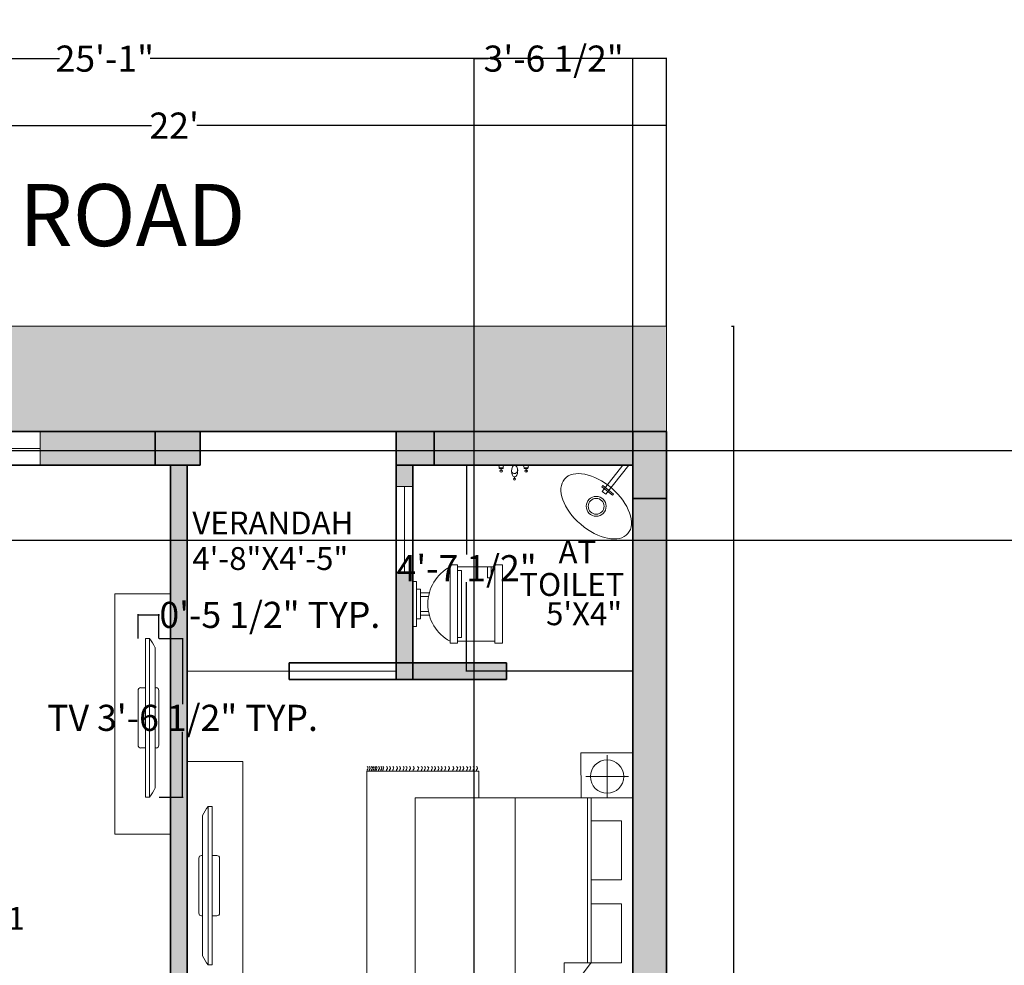
# Model space of a CAD drawing. Units: inches. Extents: x -17 to 892, y -721 to 172.
# Tile 6 of 11: x 174 to 438, y -82 to 172. Entities that reach past the tile are written whole.
import ezdxf

# ---------------------------------------------------------------- set-up
doc = ezdxf.new("R2010")
doc.units = ezdxf.units.IN
doc.header["$MEASUREMENT"] = 0
doc.layers.get('0').update_dxf_attribs({"color": 14})
for name, color, linetype, lineweight in [('A-ANNO-DIMS', 2, 'Continuous', 18), ('A-ANNO-TEXT', 7, 'Continuous', 18), ('A-AREA-IDEN', 7, 'Continuous', 18), ('A-COLS', 252, 'Continuous', 35), ('A-EQPM', 8, 'Continuous', 18), ('A-FLOR-CASE', 252, 'Continuous', 18), ('A-FLOR-FIXT', 8, 'Continuous', 18), ('A-WALL-PATT', 14, 'Continuous', 13), ('C-ROAD', 8, 'Continuous', 18), ('doors', 4, 'Continuous', 18), ('furniture', 252, 'Continuous', 18), ('walls', 252, 'Continuous', 35), ('windows', 161, 'Continuous', 18)]:
    doc.layers.add(name, color=color, linetype=linetype, lineweight=lineweight)
doc.layers.add('A-COLS-PATT', color=254, linetype='Continuous', lineweight=13, true_color=0xd7ebd2)
doc.layers.add('C-ROAD-PATT', color=9, linetype='Continuous', lineweight=13, true_color=0xafd9aa)
doc.styles.get("Standard").update_dxf_attribs({"font": 'arial.ttf'})
doc.dimstyles.get("Standard").update_dxf_attribs({"dimtxt": 7, "dimasz": 0.18, "dimexe": 0.18, "dimexo": 0.0625, "dimgap": 0.09, "dimtad": 0, "dimtih": 1, "dimtoh": 1, "dimzin": 0, "dimdsep": 46, "dimlunit": 3, "dimtxsty": 'Standard', "dimcen": 0.09, "dimadec": 0, "dimazin": 0, "dimtfac": 1, "dimtofl": 0, "dimtmove": 0, "dimatfit": 3, "dimfxl": 1, "dimtolj": 1, "dimtzin": 0, "dimarcsym": 0})

# ---------------------------------------------------------------- blocks, each defined once
blk = doc.blocks.new('CARPET')
at = {"layer": 'furniture'}
for p, q in [((-51.53, -98.11), (-51.53, -55.12)), ((-51.53, -55.12), (-41.27, -55.12)), ((36, -55.12), (51.55, -55.12)), ((51.55, -55.12), (51.55, -98.11)), ((51.55, -98.11), (-51.53, -98.11))]:
    blk.add_line(p, q, dxfattribs=at)
for points, knots in [([(-53.37, -55.99), (-53.22, -55.8), (-52.9, -55.41), (-52.34, -55.8), (-51.89, -56.08), (-51.65, -55.91), (-51.53, -55.83)], [0, 0, 0, 0, 0.653278, 1.290138, 1.740457, 2.114451, 2.114451, 2.114451, 2.114451]), ([(53.37, -55.99), (53.22, -55.8), (52.9, -55.41), (52.34, -55.8), (51.89, -56.08), (51.65, -55.91), (51.53, -55.83)], [0, 0, 0, 0, 0.653278, 1.290138, 1.740457, 2.114451, 2.114451, 2.114451, 2.114451]), ([(-53.37, -57.26), (-53.22, -57.07), (-52.9, -56.67), (-52.34, -57.07), (-51.89, -57.35), (-51.65, -57.17), (-51.53, -57.1)], [0, 0, 0, 0, 0.653278, 1.290138, 1.740457, 2.114451, 2.114451, 2.114451, 2.114451]), ([(-53.37, -58.59), (-53.22, -58.4), (-52.9, -58.01), (-52.34, -58.4), (-51.89, -58.68), (-51.65, -58.5), (-51.53, -58.43)], [0, 0, 0, 0, 0.653278, 1.290138, 1.740457, 2.114451, 2.114451, 2.114451, 2.114451]), ([(-53.37, -59.78), (-53.22, -59.58), (-52.9, -59.19), (-52.34, -59.58), (-51.89, -59.86), (-51.65, -59.69), (-51.53, -59.61)], [0, 0, 0, 0, 0.653278, 1.290138, 1.740457, 2.114451, 2.114451, 2.114451, 2.114451]), ([(53.37, -57.26), (53.22, -57.07), (52.9, -56.67), (52.34, -57.07), (51.89, -57.35), (51.65, -57.17), (51.53, -57.1)], [0, 0, 0, 0, 0.653278, 1.290138, 1.740457, 2.114451, 2.114451, 2.114451, 2.114451]), ([(53.37, -58.59), (53.22, -58.4), (52.9, -58.01), (52.34, -58.4), (51.89, -58.68), (51.65, -58.5), (51.53, -58.43)], [0, 0, 0, 0, 0.653278, 1.290138, 1.740457, 2.114451, 2.114451, 2.114451, 2.114451]), ([(53.37, -59.78), (53.22, -59.58), (52.9, -59.19), (52.34, -59.58), (51.89, -59.86), (51.65, -59.69), (51.53, -59.61)], [0, 0, 0, 0, 0.653278, 1.290138, 1.740457, 2.114451, 2.114451, 2.114451, 2.114451]), ([(-53.37, -61.22), (-53.22, -61.02), (-52.9, -60.63), (-52.34, -61.02), (-51.89, -61.3), (-51.65, -61.13), (-51.53, -61.05)], [0, 0, 0, 0, 0.653278, 1.290138, 1.740457, 2.114451, 2.114451, 2.114451, 2.114451]), ([(-53.37, -62.44), (-53.22, -62.25), (-52.9, -61.86), (-52.34, -62.25), (-51.89, -62.53), (-51.65, -62.36), (-51.53, -62.28)], [0, 0, 0, 0, 0.653278, 1.290138, 1.740457, 2.114451, 2.114451, 2.114451, 2.114451]), ([(-53.37, -63.63), (-53.22, -63.43), (-52.9, -63.04), (-52.34, -63.43), (-51.89, -63.72), (-51.65, -63.54), (-51.53, -63.46)], [0, 0, 0, 0, 0.653278, 1.290138, 1.740457, 2.114451, 2.114451, 2.114451, 2.114451]), ([(53.37, -61.22), (53.22, -61.02), (52.9, -60.63), (52.34, -61.02), (51.89, -61.3), (51.65, -61.13), (51.53, -61.05)], [0, 0, 0, 0, 0.653278, 1.290138, 1.740457, 2.114451, 2.114451, 2.114451, 2.114451]), ([(53.37, -62.44), (53.22, -62.25), (52.9, -61.86), (52.34, -62.25), (51.89, -62.53), (51.65, -62.36), (51.53, -62.28)], [0, 0, 0, 0, 0.653278, 1.290138, 1.740457, 2.114451, 2.114451, 2.114451, 2.114451]), ([(53.37, -63.63), (53.22, -63.43), (52.9, -63.04), (52.34, -63.43), (51.89, -63.72), (51.65, -63.54), (51.53, -63.46)], [0, 0, 0, 0, 0.653278, 1.290138, 1.740457, 2.114451, 2.114451, 2.114451, 2.114451]), ([(-53.37, -65.07), (-53.22, -64.87), (-52.9, -64.48), (-52.34, -64.87), (-51.89, -65.15), (-51.65, -64.98), (-51.53, -64.9)], [0, 0, 0, 0, 0.653278, 1.290138, 1.740457, 2.114451, 2.114451, 2.114451, 2.114451]), ([(-53.37, -66.76), (-53.22, -66.56), (-52.9, -66.17), (-52.34, -66.56), (-51.89, -66.84), (-51.65, -66.67), (-51.53, -66.59)], [0, 0, 0, 0, 0.653278, 1.290138, 1.740457, 2.114451, 2.114451, 2.114451, 2.114451]), ([(-53.37, -68.2), (-53.22, -68), (-52.9, -67.61), (-52.34, -68), (-51.89, -68.28), (-51.65, -68.11), (-51.53, -68.03)], [0, 0, 0, 0, 0.653278, 1.290138, 1.740457, 2.114451, 2.114451, 2.114451, 2.114451]), ([(53.37, -65.07), (53.22, -64.87), (52.9, -64.48), (52.34, -64.87), (51.89, -65.15), (51.65, -64.98), (51.53, -64.9)], [0, 0, 0, 0, 0.653278, 1.290138, 1.740457, 2.114451, 2.114451, 2.114451, 2.114451]), ([(53.37, -66.76), (53.22, -66.56), (52.9, -66.17), (52.34, -66.56), (51.89, -66.84), (51.65, -66.67), (51.53, -66.59)], [0, 0, 0, 0, 0.653278, 1.290138, 1.740457, 2.114451, 2.114451, 2.114451, 2.114451]), ([(53.37, -68.2), (53.22, -68), (52.9, -67.61), (52.34, -68), (51.89, -68.28), (51.65, -68.11), (51.53, -68.03)], [0, 0, 0, 0, 0.653278, 1.290138, 1.740457, 2.114451, 2.114451, 2.114451, 2.114451]), ([(-53.37, -69.53), (-53.22, -69.33), (-52.9, -68.94), (-52.34, -69.33), (-51.89, -69.61), (-51.65, -69.44), (-51.53, -69.36)], [0, 0, 0, 0, 0.653278, 1.290138, 1.740457, 2.114451, 2.114451, 2.114451, 2.114451]), ([(-53.37, -70.79), (-53.22, -70.6), (-52.9, -70.21), (-52.34, -70.6), (-51.89, -70.88), (-51.65, -70.7), (-51.53, -70.63)], [0, 0, 0, 0, 0.653278, 1.290138, 1.740457, 2.114451, 2.114451, 2.114451, 2.114451]), ([(-53.37, -72.12), (-53.22, -71.93), (-52.9, -71.54), (-52.34, -71.93), (-51.89, -72.21), (-51.65, -72.04), (-51.53, -71.96)], [0, 0, 0, 0, 0.653278, 1.290138, 1.740457, 2.114451, 2.114451, 2.114451, 2.114451]), ([(53.37, -69.53), (53.22, -69.33), (52.9, -68.94), (52.34, -69.33), (51.89, -69.61), (51.65, -69.44), (51.53, -69.36)], [0, 0, 0, 0, 0.653278, 1.290138, 1.740457, 2.114451, 2.114451, 2.114451, 2.114451]), ([(53.37, -70.79), (53.22, -70.6), (52.9, -70.21), (52.34, -70.6), (51.89, -70.88), (51.65, -70.7), (51.53, -70.63)], [0, 0, 0, 0, 0.653278, 1.290138, 1.740457, 2.114451, 2.114451, 2.114451, 2.114451]), ([(53.37, -72.12), (53.22, -71.93), (52.9, -71.54), (52.34, -71.93), (51.89, -72.21), (51.65, -72.04), (51.53, -71.96)], [0, 0, 0, 0, 0.653278, 1.290138, 1.740457, 2.114451, 2.114451, 2.114451, 2.114451]), ([(-53.37, -73.31), (-53.22, -73.11), (-52.9, -72.72), (-52.34, -73.11), (-51.89, -73.4), (-51.65, -73.22), (-51.53, -73.14)], [0, 0, 0, 0, 0.653278, 1.290138, 1.740457, 2.114451, 2.114451, 2.114451, 2.114451]), ([(-53.37, -74.75), (-53.22, -74.55), (-52.9, -74.16), (-52.34, -74.55), (-51.89, -74.83), (-51.65, -74.66), (-51.53, -74.58)], [0, 0, 0, 0, 0.653278, 1.290138, 1.740457, 2.114451, 2.114451, 2.114451, 2.114451]), ([(-53.37, -75.98), (-53.22, -75.78), (-52.9, -75.39), (-52.34, -75.78), (-51.89, -76.06), (-51.65, -75.89), (-51.53, -75.81)], [0, 0, 0, 0, 0.653278, 1.290138, 1.740457, 2.114451, 2.114451, 2.114451, 2.114451]), ([(53.37, -73.31), (53.22, -73.11), (52.9, -72.72), (52.34, -73.11), (51.89, -73.4), (51.65, -73.22), (51.53, -73.14)], [0, 0, 0, 0, 0.653278, 1.290138, 1.740457, 2.114451, 2.114451, 2.114451, 2.114451]), ([(53.37, -74.75), (53.22, -74.55), (52.9, -74.16), (52.34, -74.55), (51.89, -74.83), (51.65, -74.66), (51.53, -74.58)], [0, 0, 0, 0, 0.653278, 1.290138, 1.740457, 2.114451, 2.114451, 2.114451, 2.114451]), ([(53.37, -75.98), (53.22, -75.78), (52.9, -75.39), (52.34, -75.78), (51.89, -76.06), (51.65, -75.89), (51.53, -75.81)], [0, 0, 0, 0, 0.653278, 1.290138, 1.740457, 2.114451, 2.114451, 2.114451, 2.114451]), ([(-53.37, -77.16), (-53.22, -76.96), (-52.9, -76.57), (-52.34, -76.96), (-51.89, -77.25), (-51.65, -77.07), (-51.53, -76.99)], [0, 0, 0, 0, 0.653278, 1.290138, 1.740457, 2.114451, 2.114451, 2.114451, 2.114451]), ([(-53.37, -78.6), (-53.22, -78.4), (-52.9, -78.01), (-52.34, -78.4), (-51.89, -78.68), (-51.65, -78.51), (-51.53, -78.43)], [0, 0, 0, 0, 0.653278, 1.290138, 1.740457, 2.114451, 2.114451, 2.114451, 2.114451]), ([(53.37, -77.16), (53.22, -76.96), (52.9, -76.57), (52.34, -76.96), (51.89, -77.25), (51.65, -77.07), (51.53, -76.99)], [0, 0, 0, 0, 0.653278, 1.290138, 1.740457, 2.114451, 2.114451, 2.114451, 2.114451]), ([(53.37, -78.6), (53.22, -78.4), (52.9, -78.01), (52.34, -78.4), (51.89, -78.68), (51.65, -78.51), (51.53, -78.43)], [0, 0, 0, 0, 0.653278, 1.290138, 1.740457, 2.114451, 2.114451, 2.114451, 2.114451]), ([(-53.37, -80.29), (-53.22, -80.09), (-52.9, -79.7), (-52.34, -80.09), (-51.89, -80.37), (-51.65, -80.2), (-51.53, -80.12)], [0, 0, 0, 0, 0.653278, 1.290138, 1.740457, 2.114451, 2.114451, 2.114451, 2.114451]), ([(-53.37, -81.73), (-53.22, -81.53), (-52.9, -81.14), (-52.34, -81.53), (-51.89, -81.81), (-51.65, -81.64), (-51.53, -81.56)], [0, 0, 0, 0, 0.653278, 1.290138, 1.740457, 2.114451, 2.114451, 2.114451, 2.114451]), ([(-53.37, -83.06), (-53.22, -82.86), (-52.9, -82.47), (-52.34, -82.86), (-51.89, -83.14), (-51.65, -82.97), (-51.53, -82.89)], [0, 0, 0, 0, 0.653278, 1.290138, 1.740457, 2.114451, 2.114451, 2.114451, 2.114451]), ([(53.37, -80.29), (53.22, -80.09), (52.9, -79.7), (52.34, -80.09), (51.89, -80.37), (51.65, -80.2), (51.53, -80.12)], [0, 0, 0, 0, 0.653278, 1.290138, 1.740457, 2.114451, 2.114451, 2.114451, 2.114451]), ([(53.37, -81.73), (53.22, -81.53), (52.9, -81.14), (52.34, -81.53), (51.89, -81.81), (51.65, -81.64), (51.53, -81.56)], [0, 0, 0, 0, 0.653278, 1.290138, 1.740457, 2.114451, 2.114451, 2.114451, 2.114451]), ([(53.37, -83.06), (53.22, -82.86), (52.9, -82.47), (52.34, -82.86), (51.89, -83.14), (51.65, -82.97), (51.53, -82.89)], [0, 0, 0, 0, 0.653278, 1.290138, 1.740457, 2.114451, 2.114451, 2.114451, 2.114451]), ([(-53.37, -84.18), (-53.22, -83.99), (-52.9, -83.6), (-52.34, -83.99), (-51.89, -84.27), (-51.65, -84.09), (-51.53, -84.02)], [0, 0, 0, 0, 0.653278, 1.290138, 1.740457, 2.114451, 2.114451, 2.114451, 2.114451]), ([(-53.37, -85.51), (-53.22, -85.32), (-52.9, -84.93), (-52.34, -85.32), (-51.89, -85.6), (-51.65, -85.42), (-51.53, -85.35)], [0, 0, 0, 0, 0.653278, 1.290138, 1.740457, 2.114451, 2.114451, 2.114451, 2.114451]), ([(-53.37, -86.7), (-53.22, -86.5), (-52.9, -86.11), (-52.34, -86.5), (-51.89, -86.78), (-51.65, -86.61), (-51.53, -86.53)], [0, 0, 0, 0, 0.653278, 1.290138, 1.740457, 2.114451, 2.114451, 2.114451, 2.114451]), ([(53.37, -84.18), (53.22, -83.99), (52.9, -83.6), (52.34, -83.99), (51.89, -84.27), (51.65, -84.09), (51.53, -84.02)], [0, 0, 0, 0, 0.653278, 1.290138, 1.740457, 2.114451, 2.114451, 2.114451, 2.114451]), ([(53.37, -85.51), (53.22, -85.32), (52.9, -84.93), (52.34, -85.32), (51.89, -85.6), (51.65, -85.42), (51.53, -85.35)], [0, 0, 0, 0, 0.653278, 1.290138, 1.740457, 2.114451, 2.114451, 2.114451, 2.114451]), ([(53.37, -86.7), (53.22, -86.5), (52.9, -86.11), (52.34, -86.5), (51.89, -86.78), (51.65, -86.61), (51.53, -86.53)], [0, 0, 0, 0, 0.653278, 1.290138, 1.740457, 2.114451, 2.114451, 2.114451, 2.114451]), ([(-53.37, -88.14), (-53.22, -87.94), (-52.9, -87.55), (-52.34, -87.94), (-51.89, -88.22), (-51.65, -88.05), (-51.53, -87.97)], [0, 0, 0, 0, 0.653278, 1.290138, 1.740457, 2.114451, 2.114451, 2.114451, 2.114451]), ([(-53.37, -89.36), (-53.22, -89.17), (-52.9, -88.78), (-52.34, -89.17), (-51.89, -89.45), (-51.65, -89.28), (-51.53, -89.2)], [0, 0, 0, 0, 0.653278, 1.290138, 1.740457, 2.114451, 2.114451, 2.114451, 2.114451]), ([(-53.37, -90.55), (-53.22, -90.35), (-52.9, -89.96), (-52.34, -90.35), (-51.89, -90.64), (-51.65, -90.46), (-51.53, -90.38)], [0, 0, 0, 0, 0.653278, 1.290138, 1.740457, 2.114451, 2.114451, 2.114451, 2.114451]), ([(53.37, -88.14), (53.22, -87.94), (52.9, -87.55), (52.34, -87.94), (51.89, -88.22), (51.65, -88.05), (51.53, -87.97)], [0, 0, 0, 0, 0.653278, 1.290138, 1.740457, 2.114451, 2.114451, 2.114451, 2.114451]), ([(53.37, -89.36), (53.22, -89.17), (52.9, -88.78), (52.34, -89.17), (51.89, -89.45), (51.65, -89.28), (51.53, -89.2)], [0, 0, 0, 0, 0.653278, 1.290138, 1.740457, 2.114451, 2.114451, 2.114451, 2.114451]), ([(53.37, -90.55), (53.22, -90.35), (52.9, -89.96), (52.34, -90.35), (51.9, -90.63), (51.66, -90.47), (51.55, -90.4)], [0, 0, 0, 0, 0.653278, 1.290138, 1.740457, 2.0926, 2.0926, 2.0926, 2.0926]), ([(-53.37, -91.99), (-53.22, -91.79), (-52.9, -91.4), (-52.34, -91.79), (-51.89, -92.07), (-51.65, -91.9), (-51.53, -91.82)], [0, 0, 0, 0, 0.653278, 1.290138, 1.740457, 2.114451, 2.114451, 2.114451, 2.114451]), ([(-53.37, -92.69), (-53.22, -92.48), (-52.9, -92.08), (-52.35, -92.49), (-51.89, -92.77), (-51.65, -92.6), (-51.53, -92.52)], [0, 0, 0, 0, 0.663904, 1.307406, 1.757725, 2.131719, 2.131719, 2.131719, 2.131719]), ([(-53.37, -93.61), (-53.22, -93.42), (-52.9, -93.03), (-52.34, -93.42), (-51.89, -93.7), (-51.65, -93.52), (-51.53, -93.45)], [0, 0, 0, 0, 0.653278, 1.290138, 1.740457, 2.114451, 2.114451, 2.114451, 2.114451]), ([(-53.37, -94.55), (-53.22, -94.35), (-52.9, -93.96), (-52.34, -94.35), (-51.89, -94.63), (-51.65, -94.46), (-51.53, -94.38)], [0, 0, 0, 0, 0.653278, 1.290138, 1.740457, 2.114451, 2.114451, 2.114451, 2.114451]), ([(53.37, -91.99), (53.22, -91.79), (52.9, -91.4), (52.34, -91.79), (51.9, -92.07), (51.66, -91.91), (51.55, -91.83)], [0, 0, 0, 0, 0.653278, 1.290138, 1.740457, 2.0926, 2.0926, 2.0926, 2.0926]), ([(53.37, -92.69), (53.22, -92.49), (52.9, -92.09), (52.34, -92.49), (51.9, -92.77), (51.66, -92.61), (51.55, -92.53)], [0, 0, 0, 0, 0.656792, 1.295826, 1.746145, 2.098292, 2.098292, 2.098292, 2.098292]), ([(53.37, -93.66), (53.22, -93.46), (52.9, -93.07), (52.34, -93.46), (51.9, -93.74), (51.66, -93.58), (51.55, -93.5)], [0, 0, 0, 0, 0.653278, 1.290138, 1.740457, 2.0926, 2.0926, 2.0926, 2.0926]), ([(53.37, -94.59), (53.22, -94.4), (52.9, -94.01), (52.34, -94.4), (51.9, -94.68), (51.66, -94.51), (51.55, -94.44)], [0, 0, 0, 0, 0.653278, 1.290138, 1.740457, 2.0926, 2.0926, 2.0926, 2.0926]), ([(-53.37, -95.05), (-53.22, -94.85), (-52.9, -94.46), (-52.34, -94.85), (-51.89, -95.14), (-51.65, -94.96), (-51.53, -94.88)], [0, 0, 0, 0, 0.653278, 1.290138, 1.740457, 2.114451, 2.114451, 2.114451, 2.114451]), ([(-53.37, -95.73), (-53.22, -95.54), (-52.9, -95.15), (-52.34, -95.54), (-51.89, -95.82), (-51.65, -95.65), (-51.53, -95.57)], [0, 0, 0, 0, 0.653278, 1.290138, 1.740457, 2.114451, 2.114451, 2.114451, 2.114451]), ([(-53.37, -96.38), (-53.22, -96.18), (-52.9, -95.79), (-52.34, -96.18), (-51.89, -96.47), (-51.65, -96.29), (-51.53, -96.21)], [0, 0, 0, 0, 0.653278, 1.290138, 1.740457, 2.114451, 2.114451, 2.114451, 2.114451]), ([(-53.37, -97.17), (-53.22, -96.98), (-52.9, -96.59), (-52.34, -96.98), (-51.89, -97.26), (-51.65, -97.08), (-51.53, -97.01)], [0, 0, 0, 0, 0.653278, 1.290138, 1.740457, 2.114451, 2.114451, 2.114451, 2.114451]), ([(-53.37, -97.99), (-53.22, -97.79), (-52.9, -97.4), (-52.34, -97.79), (-51.89, -98.08), (-51.65, -97.9), (-51.53, -97.82)], [0, 0, 0, 0, 0.653278, 1.290138, 1.740457, 2.114451, 2.114451, 2.114451, 2.114451]), ([(53.37, -95.78), (53.22, -95.58), (52.9, -95.19), (52.34, -95.58), (51.89, -95.86), (51.65, -95.69), (51.53, -95.61)], [0, 0, 0, 0, 0.653278, 1.290138, 1.740457, 2.114451, 2.114451, 2.114451, 2.114451]), ([(53.37, -96.43), (53.22, -96.23), (52.9, -95.84), (52.34, -96.23), (51.89, -96.51), (51.65, -96.34), (51.53, -96.26)], [0, 0, 0, 0, 0.653278, 1.290138, 1.740457, 2.114451, 2.114451, 2.114451, 2.114451]), ([(53.37, -97.22), (53.22, -97.02), (52.9, -96.63), (52.34, -97.02), (51.89, -97.3), (51.65, -97.13), (51.53, -97.05)], [0, 0, 0, 0, 0.653278, 1.290138, 1.740457, 2.114451, 2.114451, 2.114451, 2.114451]), ([(53.37, -97.99), (53.22, -97.79), (52.9, -97.4), (52.34, -97.79), (51.89, -98.08), (51.65, -97.9), (51.53, -97.82)], [0, 0, 0, 0, 0.653278, 1.290138, 1.740457, 2.114451, 2.114451, 2.114451, 2.114451]), ([(53.37, -95.1), (53.22, -94.9), (52.9, -94.51), (52.34, -94.9), (51.9, -95.18), (51.66, -95.02), (51.55, -94.94)], [0, 0, 0, 0, 0.653278, 1.290138, 1.740457, 2.0926, 2.0926, 2.0926, 2.0926])]:
    blk.add_open_spline(points, degree=3, knots=knots, dxfattribs=at)
blk = doc.blocks.new('A$C58D270C6')
at = {"layer": 'furniture'}
for p, q in [((9.09, 124.13), (9.09, 108.87)), ((1.46, 116.5), (16.73, 116.5)), ((14.97, 94.84), (24.62, 107.92)), ((24.62, 94.93), (24.62, 107.92)), ((42.08, 108), (42.08, 36)), ((14.97, 94.93), (24.62, 94.93)), ((14.97, 94.84), (14.97, 36)), ((16.22, 94.93), (16.22, 36)), ((9.25, 36), (9.25, 20.74)), ((1.62, 28.37), (16.88, 28.37))]:
    blk.add_line(p, q, dxfattribs=at)
for points in [[(18.5, 108), (18.34, 124.13), (-0.16, 124.13), (0, 108)], [(0, 108), (77.91, 108), (77.91, 36), (0, 36)], [(4.09, 94.93), (14.97, 94.93), (14.97, 73.83), (4.09, 73.83)], [(4.09, 65.23), (14.97, 65.23), (14.97, 44.13), (4.09, 44.13)], [(18.65, 19.87), (18.5, 36), (0, 36), (0.16, 19.87)]]:
    blk.add_lwpolyline(points, close=True, dxfattribs=at)
for centre in [(9.09, 116.5), (9.25, 28.37)]:
    blk.add_circle(centre, 5.95, dxfattribs=at)
at = {"layer": 'furniture', "xscale": 0.9312884925094044, "yscale": 0.9312884925094044, "zscale": 0.9312884925094044, "rotation": 90}
blk.add_blockref('CARPET', (3.79, 74.47), dxfattribs=at)
blk = doc.blocks.new('PLASMA-LARGE')
at = {"layer": 'furniture'}
for p, q in [((-7.26, 0), (7.26, 0)), ((-21, -2.5), (21, -2.5)), ((-21, -2.5), (-21, -3.5)), ((-18.61, -1), (18.61, -1)), ((-8, -1), (-8, -0.74)), ((8, -1), (8, -0.74)), ((21, -2.5), (21, -3.5)), ((-21, -3.5), (21, -3.5)), ((-8, -3.5), (-8, -4.76)), ((8, -3.5), (8, -4.76)), ((-7.26, -5.5), (7.26, -5.5))]:
    blk.add_line(p, q, dxfattribs=at)
for centre, radius, start, end in [((-7.26, -0.74), 0.744, 90, 180), ((7.26, -0.74), 0.744, 0, 90), ((-13.97, -11.05), 11.07, 114.7602, 129.4175), ((13.97, -11.05), 11.07, 50.5825, 65.2398), ((-7.26, -4.76), 0.744, 180, 270), ((7.26, -4.76), 0.744, 270, 0)]:
    blk.add_arc(centre, radius, start, end, dxfattribs=at)
blk = doc.blocks.new('*U12')
for p, q in [((-10, 22), (-10, 12)), ((10, 12), (10, 22)), ((-10, 21), (-7, 21)), ((-7, 20), (-10, 20)), ((-7, 21), (-7, 20)), ((10.5, 12), (-10.5, 12)), ((-10.5, 10), (-10.5, 12)), ((9, 13), (-9, 13)), ((-9, 13), (-9, 12)), ((9, 12), (9, 13)), ((10.5, 12), (10.5, 10)), ((10.5, 10), (-10.5, 10)), ((-3, 4.4065), (-3, 2)), ((-2, 2), (-2, 4.1658)), ((2, 4.1658), (2, 2)), ((3, 2), (3, 4.4065)), ((4, 2), (-4, 2)), ((-4, 2), (-4, 1)), ((4, 1), (4, 2))]:
    blk.add_line(p, q)
for points in [[(10.5, 22), (10.5, 24), (-10.5, 24), (-10.5, 22)], [(6, 0), (6, 1), (-6, 1), (-6, 0)]]:
    blk.add_lwpolyline(points, close=True)
blk.add_arc((0, 15.3333), 11.3333, 208.0725, 331.9275)
blk = doc.blocks.new('*D15')
at = {"layer": 'A-ANNO-DIMS', "color": 0, "lineweight": -2, "transparency": 16777216}
for p, q in [((83.08, 142.49), (83.08, 143.87)), ((83.26, 143.69), (208.99, 143.69)), ((346.9, 143.69), (221.17, 143.69)), ((347.08, 142.49), (347.08, 143.87))]:
    blk.add_line(p, q, dxfattribs=at)
at = {"layer": 'A-ANNO-DIMS', "color": 0, "lineweight": 100, "transparency": 16777216}
for points in [[(83.26, 143.72), (83.26, 143.66), (83.08, 143.69)], [(346.9, 143.72), (346.9, 143.66), (347.08, 143.69)]]:
    blk.add_solid(points, dxfattribs=at)
at = {"layer": 'Defpoints', "color": 0, "lineweight": 100, "transparency": 16777216}
for p in [(347.08, 143.69), (83.08, 142.43), (347.08, 142.43)]:
    blk.add_point(p, dxfattribs=at)
at = {"layer": 'A-ANNO-DIMS', "color": 0, "transparency": 16777216, "insert": (215.08, 143.69), "char_height": 7, "attachment_point": 5}
blk.add_mtext("\\A1;22'", dxfattribs=at)
blk = doc.blocks.new('*D16')
at = {"layer": 'A-ANNO-DIMS', "color": 0, "lineweight": -2, "transparency": 16777216}
for p, q in [((364.49, 89.9), (365.24, 89.9)), ((365.06, 89.72), (365.06, -263.08)), ((365.06, -623.21), (365.06, -270.41)), ((364.49, -623.39), (365.24, -623.39))]:
    blk.add_line(p, q, dxfattribs=at)
at = {"layer": 'A-ANNO-DIMS', "color": 0, "lineweight": 100, "transparency": 16777216}
for points in [[(365.03, 89.72), (365.09, 89.72), (365.06, 89.9)], [(365.03, -623.21), (365.09, -623.21), (365.06, -623.39)]]:
    blk.add_solid(points, dxfattribs=at)
at = {"layer": 'Defpoints', "color": 0, "lineweight": 100, "transparency": 16777216}
for p in [(364.43, 89.9), (364.43, -623.39), (365.06, -623.39)]:
    blk.add_point(p, dxfattribs=at)
at = {"layer": 'A-ANNO-DIMS', "color": 0, "transparency": 16777216, "insert": (365.06, -266.74), "char_height": 7, "attachment_point": 5}
blk.add_mtext('\\A1;57\'-1"', dxfattribs=at)
blk = doc.blocks.new('WIN-68-INSET')
for p, q in [((0, 9), (0, 0)), ((0, 9), (0, 4.5)), ((67.89, 0), (67.89, 9)), ((0, 4.5), (67.89, 4.5))]:
    blk.add_line(p, q)
blk = doc.blocks.new('BASIN-CORNER')
for p, q in [((11.05, 12.77), (16.6, 19.78)), ((18.18, 19.78), (12.02, 12)), ((11.25, 14.32), (11, 14)), ((11, 14), (13.87, 11.73)), ((14.12, 12.04), (11.25, 14.32)), ((12.02, 12), (11.05, 12.77)), ((13.87, 11.73), (14.12, 12.05))]:
    blk.add_line(p, q)
for radius in [2.67, 2.13, 2.13, 2.13]:
    blk.add_circle((9.46, 8.76), radius)
blk.add_ellipse((9.46, 8.76), major_axis=(-8.49, 7.31), ratio=0.56899)
blk = doc.blocks.new('MEDIA-CONSOLE')
for p, q in [((14.9, 64.44), (0, 64.44)), ((14.9, 0), (14.9, 64.44)), ((0, 0), (14.9, 0))]:
    blk.add_line(p, q)
blk = doc.blocks.new('*D32')
at = {"layer": 'A-ANNO-DIMS', "color": 0, "lineweight": -2, "transparency": 16777216}
for p, q in [((211.04, 6.1), (217.52, 6.1)), ((217.34, 5.92), (217.34, -11.43)), ((217.34, -36.2), (217.34, -18.85)), ((211.04, -36.38), (217.52, -36.38))]:
    blk.add_line(p, q, dxfattribs=at)
at = {"layer": 'A-ANNO-DIMS', "color": 0, "lineweight": 100, "transparency": 16777216}
for points in [[(217.31, 5.92), (217.37, 5.92), (217.34, 6.1)], [(217.31, -36.2), (217.37, -36.2), (217.34, -36.38)]]:
    blk.add_solid(points, dxfattribs=at)
at = {"layer": 'Defpoints', "color": 0, "lineweight": 100, "transparency": 16777216}
for p in [(210.97, 6.1), (210.97, -36.38), (217.34, -36.38)]:
    blk.add_point(p, dxfattribs=at)
at = {"layer": 'A-ANNO-DIMS', "color": 0, "transparency": 16777216, "insert": (217.34, -15.14), "char_height": 7, "attachment_point": 5}
blk.add_mtext('\\A1;TV 3\'-6 1/2" TYP.', dxfattribs=at)
blk = doc.blocks.new('*D33')
at = {"layer": 'A-ANNO-DIMS', "color": 0, "lineweight": -2, "transparency": 16777216}
for p, q in [((205.41, 6.16), (205.41, 12.65)), ((205.59, 12.47), (210.79, 12.47)), ((210.97, 6.16), (210.97, 12.65)), ((210.97, 12.47), (211.15, 12.47))]:
    blk.add_line(p, q, dxfattribs=at)
at = {"layer": 'A-ANNO-DIMS', "color": 0, "lineweight": 100, "transparency": 16777216}
for points in [[(205.59, 12.5), (205.59, 12.44), (205.41, 12.47)], [(210.79, 12.5), (210.79, 12.44), (210.97, 12.47)]]:
    blk.add_solid(points, dxfattribs=at)
at = {"layer": 'Defpoints', "color": 0, "lineweight": 100, "transparency": 16777216}
for p in [(210.97, 12.47), (205.41, 6.1), (210.97, 6.1)]:
    blk.add_point(p, dxfattribs=at)
at = {"layer": 'A-ANNO-DIMS', "color": 0, "transparency": 16777216, "insert": (240.73, 12.47), "char_height": 7, "attachment_point": 5}
blk.add_mtext('\\A1;0\'-5 1/2" TYP.', dxfattribs=at)
blk = doc.blocks.new('*D56')
at = {"layer": 'A-ANNO-DIMS', "color": 0, "lineweight": -2, "transparency": 16777216}
for p, q in [((45.89, 61.67), (45.89, 161.84)), ((46.07, 161.66), (184.32, 161.66)), ((346.9, 161.66), (208.66, 161.66)), ((347.08, 89.96), (347.08, 161.84))]:
    blk.add_line(p, q, dxfattribs=at)
at = {"layer": 'A-ANNO-DIMS', "color": 0, "lineweight": 100, "transparency": 16777216}
for points in [[(46.07, 161.69), (46.07, 161.63), (45.89, 161.66)], [(346.9, 161.69), (346.9, 161.63), (347.08, 161.66)]]:
    blk.add_solid(points, dxfattribs=at)
at = {"layer": 'Defpoints', "color": 0, "lineweight": 100, "transparency": 16777216}
for p in [(45.89, 161.66), (347.08, 89.9), (45.89, 61.61)]:
    blk.add_point(p, dxfattribs=at)
at = {"layer": 'A-ANNO-DIMS', "color": 0, "transparency": 16777216, "insert": (196.49, 161.66), "char_height": 7, "attachment_point": 5}
blk.add_mtext('\\A1;25\'-1"', dxfattribs=at)
blk = doc.blocks.new('*D63')
at = {"layer": 'A-ANNO-DIMS', "color": 0, "lineweight": -2, "transparency": 16777216}
for p, q in [((295.55, -619.99), (295.55, 161.84)), ((295.73, 161.66), (299.27, 161.66)), ((337.9, 161.66), (334.36, 161.66)), ((338.08, -619.99), (338.08, 161.84))]:
    blk.add_line(p, q, dxfattribs=at)
at = {"layer": 'A-ANNO-DIMS', "color": 0, "lineweight": 100, "transparency": 16777216}
for points in [[(295.73, 161.69), (295.73, 161.63), (295.55, 161.66)], [(337.9, 161.69), (337.9, 161.63), (338.08, 161.66)]]:
    blk.add_solid(points, dxfattribs=at)
at = {"layer": 'Defpoints', "color": 0, "lineweight": 100, "transparency": 16777216}
for p in [(338.08, 161.66), (295.55, -620.06), (338.08, -620.06)]:
    blk.add_point(p, dxfattribs=at)
at = {"layer": 'A-ANNO-DIMS', "color": 0, "transparency": 16777216, "insert": (316.82, 161.66), "char_height": 7, "attachment_point": 5}
blk.add_mtext('\\A1;3\'-6 1/2"', dxfattribs=at)
blk = doc.blocks.new('*D68')
at = {"layer": 'A-ANNO-DIMS', "color": 0, "lineweight": -2, "transparency": 16777216}
for p, q in [((738.65, 56.46), (1.11, 56.46)), ((1.29, 56.28), (1.29, 48.13)), ((1.29, 32.64), (1.29, 40.8)), ((737.65, 32.46), (1.11, 32.46))]:
    blk.add_line(p, q, dxfattribs=at)
at = {"layer": 'A-ANNO-DIMS', "color": 0, "lineweight": 100, "transparency": 16777216}
for points in [[(1.26, 56.28), (1.32, 56.28), (1.29, 56.46)], [(1.26, 32.64), (1.32, 32.64), (1.29, 32.46)]]:
    blk.add_solid(points, dxfattribs=at)
at = {"layer": 'Defpoints', "color": 0, "lineweight": 100, "transparency": 16777216}
for p in [(738.71, 56.46), (1.29, 32.46), (737.71, 32.46)]:
    blk.add_point(p, dxfattribs=at)
at = {"layer": 'A-ANNO-DIMS', "color": 0, "transparency": 16777216, "insert": (1.29, 44.46), "char_height": 7, "attachment_point": 5}
blk.add_mtext('\\A1;2\'-0"', dxfattribs=at)
blk = doc.blocks.new('*D69')
at = {"layer": 'A-ANNO-DIMS', "color": 0, "lineweight": -2, "transparency": 16777216}
for p, q in [((338.02, 52.61), (293.3, 52.61)), ((293.48, 52.43), (293.48, 28.7)), ((293.48, -2.46), (293.48, 21.28)), ((338.02, -2.64), (293.3, -2.64))]:
    blk.add_line(p, q, dxfattribs=at)
at = {"layer": 'A-ANNO-DIMS', "color": 0, "lineweight": 100, "transparency": 16777216}
for points in [[(293.45, 52.43), (293.51, 52.43), (293.48, 52.61)], [(293.45, -2.46), (293.51, -2.46), (293.48, -2.64)]]:
    blk.add_solid(points, dxfattribs=at)
at = {"layer": 'Defpoints', "color": 0, "lineweight": 100, "transparency": 16777216}
for p in [(293.48, 52.61), (338.08, 52.61), (338.08, -2.64)]:
    blk.add_point(p, dxfattribs=at)
at = {"layer": 'A-ANNO-DIMS', "color": 0, "transparency": 16777216, "insert": (293.48, 24.99), "char_height": 7, "attachment_point": 5}
blk.add_mtext('\\A1;4\'-7 1/2"', dxfattribs=at)

msp = doc.modelspace()

# ---------------------------------------------------------------- hatches: boundary and pattern name
at = {"layer": 'A-COLS-PATT'}
h = msp.add_hatch(color=256, dxfattribs=at)
h.dxf.hatch_style = 1
h.paths.add_polyline_path([(92.084, 61.611), (83.084, 61.611), (83.084, 43.692), (92.084, 43.692)])
h.paths.add_polyline_path([(347.084, 61.611), (338.084, 61.611), (338.084, 43.692), (347.084, 43.692)])
h.paths.add_polyline_path([(222.053, 61.611), (209.95, 61.611), (209.95, 52.611), (222.053, 52.611)])
h.paths.add_polyline_path([(284.798, 61.611), (274.584, 61.611), (274.584, 52.611), (284.798, 52.611)])
h.paths.add_polyline_path([(223.084, -106.389), (214.084, -106.389), (214.084, -119.959), (223.084, -119.959)])
h.paths.add_polyline_path([(347.084, -148.653), (338.084, -148.653), (338.084, -172.24), (347.084, -172.24)])
h.paths.add_polyline_path([(92.084, -102.402), (83.084, -102.402), (83.084, -119.959), (92.084, -119.959)])
h.paths.add_polyline_path([(92.084, -205.889), (83.084, -205.889), (83.084, -216.319), (92.084, -216.319)])
h.paths.add_polyline_path([(347.084, -349.073), (338.084, -349.073), (338.084, -372.66), (347.084, -372.66)])
h.paths.add_polyline_path([(347.084, -610.134), (338.084, -610.134), (338.084, -614.389), (338.084, -623.342), (347.084, -623.342)])
h.paths.add_polyline_path([(221.166, -610.357), (214.084, -610.357), (214.084, -623.389), (219.084, -623.389), (221.166, -623.389), (221.166, -621.723)])
h.paths.add_polyline_path([(90.166, -610.357), (83.084, -610.357), (83.084, -623.389), (90.166, -623.389)])
h.paths.add_polyline_path([(223.084, -401.64), (214.084, -401.64), (214.084, -410.389), (223.084, -410.389)])
h.paths.add_polyline_path([(223.084, -356.889), (214.084, -356.889), (214.084, -369.273), (223.084, -369.273)])
h.paths.add_polyline_path([(92.084, -398.492), (83.084, -398.492), (83.084, -410.389), (92.084, -410.389)])
h.paths.add_polyline_path([(92.084, -348.918), (83.084, -348.918), (83.084, -360.706), (92.084, -360.706)])
at = {"layer": 'A-WALL-PATT'}
h = msp.add_hatch(color=256, dxfattribs=at)
h.dxf.hatch_style = 1
h.paths.add_polyline_path([(111.26, 61.611), (92.084, 61.611), (92.084, 52.611), (111.26, 52.611)])
h.paths.add_polyline_path([(209.95, 61.611), (179.154, 61.611), (179.154, 52.611), (209.95, 52.611)])
h.paths.add_polyline_path([(338.084, 61.611), (284.798, 61.611), (284.798, 52.611), (338.084, 52.611)])
h.paths.add_polyline_path([(279.084, 23.861), (274.584, 23.861), (274.584, -0.389), (279.084, -0.389)])
h.paths.add_polyline_path([(279.084, 52.611), (274.584, 52.611), (274.584, 46.881), (276.834, 46.881), (279.084, 46.881)])
h.paths.add_polyline_path([(279.084, -0.389), (274.584, -0.389), (274.584, -4.889), (279.084, -4.889)])
h.paths.add_polyline_path([(304.22, -0.389), (279.084, -0.389), (279.084, -4.889), (304.22, -4.889)])
h.paths.add_polyline_path([(347.084, 43.692), (338.084, 43.692), (338.084, -148.653), (347.084, -148.653)])
h.paths.add_polyline_path([(338.084, -154.889), (264.103, -154.889), (264.103, -163.889), (338.084, -163.889)])
h.paths.add_polyline_path([(223.084, -119.959), (214.084, -119.959), (214.084, -163.889), (223.084, -163.889)])
h.paths.add_polyline_path([(218.584, 52.611), (214.084, 52.611), (214.084, -106.389), (218.584, -106.389)])
h.paths.add_polyline_path([(92.084, -8.943), (83.084, -8.943), (83.084, -49.69), (87.584, -49.69), (92.084, -49.69)])
h.paths.add_polyline_path([(92.084, 43.692), (83.084, 43.692), (83.084, 33.018), (87.584, 33.018), (92.084, 33.018)])
h.paths.add_polyline_path([(92.084, -91.651), (83.084, -91.651), (83.084, -102.402), (92.084, -102.402)])
h.paths.add_polyline_path([(92.084, -119.959), (83.084, -119.959), (83.084, -151.855), (87.584, -151.855), (92.084, -151.855)])
h.paths.add_polyline_path([(173.584, -108.639), (173.584, -106.389), (173.084, -106.389), (92.084, -106.389), (92.084, -110.889), (169.084, -110.889), (169.084, -176.029), (173.584, -176.029)])
h.paths.add_polyline_path([(92.084, -185.221), (83.084, -185.221), (83.084, -205.889), (92.084, -205.889)])
h.paths.add_polyline_path([(92.084, -216.319), (83.084, -216.319), (83.084, -259.015), (87.584, -259.015), (92.084, -259.015)])
h.paths.add_polyline_path([(173.584, -205.889), (92.084, -205.889), (92.084, -210.389), (169.084, -210.389), (169.084, -236.193), (173.584, -236.193)])
h.paths.add_polyline_path([(92.084, -300.976), (83.084, -300.976), (83.084, -348.918), (92.084, -348.918)])
h.paths.add_polyline_path([(87.584, -410.389), (83.084, -410.389), (83.084, -610.357), (87.584, -610.357)])
h.paths.add_polyline_path([(115.523, -614.389), (90.166, -614.389), (90.166, -623.389), (115.523, -623.389)])
h.paths.add_polyline_path([(214.084, -614.389), (174.149, -614.389), (174.149, -623.389), (214.084, -623.389)])
h.paths.add_polyline_path([(219.084, -410.389), (214.084, -410.389), (214.084, -610.357), (219.084, -610.357)])
h.paths.add_polyline_path([(347.084, -372.66), (338.084, -372.66), (338.084, -610.134), (347.084, -610.134)])
h.paths.add_polyline_path([(347.084, -172.24), (338.084, -172.24), (338.084, -349.073), (347.084, -349.073)])
h.paths.add_polyline_path([(338.084, -356.889), (317.618, -356.889), (317.618, -365.889), (338.084, -365.889)])
h.paths.add_polyline_path([(267.632, -356.889), (263.828, -356.889), (263.828, -365.889), (267.632, -365.889)])
h.paths.add_polyline_path([(223.084, -369.273), (214.084, -369.273), (214.084, -401.64), (223.084, -401.64)])
at = {"layer": 'C-ROAD-PATT'}
h = msp.add_hatch(dxfattribs=at)
h.set_pattern_fill('BRICK', color=256)
h.paths.add_polyline_path([(347.084, 89.902), (83.084, 89.902), (83.084, 61.611), (347.084, 61.611)])

# ---------------------------------------------------------------- linework, layer by layer
at = {"layer": 'A-COLS'}
for p, q in [((209.95, 52.611), (209.95, 61.611)), ((222.053, 52.611), (222.053, 61.611)), ((274.584, 52.611), (274.584, 61.611)), ((274.584, 61.611), (284.798, 61.611)), ((284.798, 61.611), (284.798, 52.611)), ((284.798, 52.611), (279.084, 52.611)), ((338.084, 43.692), (347.084, 43.692))]:
    msp.add_line(p, q, dxfattribs=at)
at = {"layer": 'A-FLOR-FIXT'}
for p, q in [((302.232, 51.929), (303.268, 51.943)), ((302.243, 51.744), (303.256, 51.744)), ((302.749, 51.744), (302.749, 51.053)), ((308.908, 51.923), (309.941, 51.926)), ((308.918, 51.744), (309.931, 51.744)), ((309.424, 51.744), (309.424, 51.053)), ((306.334, 49.471), (306.334, 48.89))]:
    msp.add_line(p, q, dxfattribs=at)
for centre, radius in [((302.749, 51.053), 0.345), ((309.424, 51.053), 0.345), ((306.334, 48.89), 0.291)]:
    msp.add_circle(centre, radius, dxfattribs=at)
for centre, radius, start, end in [((300.67, 51.744), 1.573, 0, 33.45047), ((304.828, 51.744), 1.573, 146.54953, 180), ((306.334, 51.233), 0.852, 193.058, 23.65476), ((307.345, 51.744), 1.573, 0, 33.45047), ((311.503, 51.744), 1.573, 146.54953, 180)]:
    msp.add_arc(centre, radius, start, end, dxfattribs=at)
msp.add_ellipse((306.334, 51.041), major_axis=(0, 1.57), ratio=0.5286709, dxfattribs=at)
at = {"layer": 'C-ROAD'}
for p, q in [((83.084, 89.902), (347.084, 89.902)), ((347.084, 89.902), (347.084, 61.611))]:
    msp.add_line(p, q, dxfattribs=at)
at = {"layer": 'doors'}
for p, q in [((245.879, -2.639), (218.584, -2.639)), ((304.22, -2.639), (338.084, -2.639))]:
    msp.add_line(p, q, dxfattribs=at)
at = {"layer": 'walls'}
for p, q in [((83.084, 61.611), (347.084, 61.611)), ((338.084, 61.611), (338.084, -614.389)), ((347.084, 61.611), (347.084, -623.389)), ((92.084, 52.611), (222.053, 52.611)), ((214.084, -163.889), (214.084, 52.611)), ((218.584, -106.389), (218.584, 52.611)), ((274.584, -4.889), (274.584, 52.611)), ((274.584, 52.611), (338.084, 52.611)), ((279.084, -4.889), (279.084, 52.611)), ((245.879, -0.389), (304.22, -0.389)), ((245.879, -0.389), (245.879, -4.889)), ((304.22, -0.389), (304.22, -4.889)), ((245.879, -4.889), (304.22, -4.889))]:
    msp.add_line(p, q, dxfattribs=at)
at = {"layer": 'windows'}
for p, q in [((274.584, 46.881), (279.084, 46.881)), ((274.584, 23.861), (274.584, 46.881)), ((274.584, 46.881), (276.834, 46.881)), ((276.834, 46.881), (276.834, 23.861)), ((279.084, 46.881), (279.084, 23.861)), ((279.084, 23.861), (274.584, 23.861)), ((245.879, -2.639), (245.879, -0.389)), ((245.879, -0.389), (245.879, -4.889)), ((245.879, -2.639), (274.584, -2.639)), ((274.584, -2.639), (274.584, -0.389)), ((274.584, -0.389), (274.584, -4.889))]:
    msp.add_line(p, q, dxfattribs=at)

# ---------------------------------------------------------------- block references
at = {"layer": 'A-EQPM', "yscale": 1.011294184530666, "zscale": 1.011294184530666}
for p, xscale, rotation in [((210.973, -15.14), 1.011294184530666, 270), ((221.696, -60.15), -1.011294184530666, 90)]:
    msp.add_blockref('PLASMA-LARGE', p, dxfattribs=dict(at, xscale=xscale, rotation=rotation))
at = {"layer": 'A-FLOR-CASE', "rotation": 180}
msp.add_blockref('MEDIA-CONSOLE', (214.084, 18.121), dxfattribs=at)
at = {"layer": 'A-FLOR-CASE'}
msp.add_blockref('MEDIA-CONSOLE', (218.584, -91.332), dxfattribs=at)
at = {"layer": 'A-FLOR-FIXT'}
msp.add_blockref('BASIN-CORNER', (318.772, 32.833), dxfattribs=at)
at = {"layer": 'A-FLOR-FIXT', "rotation": 270}
msp.add_blockref('*U12', (279.084, 15.386), dxfattribs=at)
at = {"layer": 'furniture', "xscale": 0.7500000390647866, "yscale": 0.7500000390647866, "zscale": 0.7500000390647866, "rotation": 180}
msp.add_blockref('A$C58D270C6', (338.084, -9.622), dxfattribs=at)
at = {"layer": 'windows'}
msp.add_blockref('WIN-68-INSET', (111.26, 52.611), dxfattribs=at)

# ---------------------------------------------------------------- texts
at = {"layer": 'A-ANNO-TEXT'}
msp.add_text('ROAD', height=16.6398, dxfattribs=at).set_placement((173.505, 111.371))
at = {"layer": 'A-AREA-IDEN'}
for s, p in [('VERANDAH', (219.969, 34.048)), ('AT', (318.128, 26.275)), ('4\'-8"X4\'-5"', (219.969, 24.513)), ('TOILET', (307.616, 17.558)), ('5\'X4"', (314.783, 9.707)), ('BEDROOM-01', (122.122, -71.994))]:
    msp.add_text(s, height=6.1361, dxfattribs=at).set_placement(p)

# ---------------------------------------------------------------- dimensions: what is measured, and where the dimension line sits
at = {"layer": 'A-ANNO-DIMS'}
for base, p1, p2, override, picture, middle in [((338.084, 161.663), (295.55, -620.057), (338.084, -620.057), {"dimdec": 1, "dimlfac": 1, "dimrnd": 0, "dimzin": 1, "dimdsep": 46, "dimlunit": 4, "dimfrac": 2}, '*D63', (316.817, 161.663)), ((45.892, 161.663), (347.084, 89.902), (45.892, 61.611), {"dimdec": 1, "dimlfac": 1, "dimrnd": 0, "dimzin": 1, "dimdsep": 46, "dimlunit": 4, "dimfrac": 2}, '*D56', (196.488, 161.663)), ((347.084, 143.692), (83.084, 142.427), (347.084, 142.427), {"dimclrd": 0, "dimclre": 0, "dimclrt": 0}, '*D15', (215.084, 143.692))]:
    dim = msp.add_linear_dim(base=base, p1=p1, p2=p2, dimstyle='Standard', override=override, dxfattribs=at)
    dim.commit()
    dim.dimension.update_dxf_attribs({"geometry": picture, "text_midpoint": middle})
for base, p1, p2, angle, text, override, picture, middle in [((365.057, -623.389), (364.432, 89.902), (364.432, -623.389), 90, '57\'-1"', {"dimclrd": 0, "dimclre": 0, "dimclrt": 0}, '*D16', (365.057, -266.744)), ((217.344, -36.378), (210.973, 6.097), (210.973, -36.378), 270, 'TV <> TYP.', {"dimdec": 1, "dimlfac": 1, "dimrnd": 0, "dimzin": 1, "dimdsep": 46, "dimlunit": 4, "dimfrac": 2}, '*D32', (217.344, -15.14))]:
    dim = msp.add_linear_dim(base=base, p1=p1, p2=p2, angle=angle, text=text, dimstyle='Standard', override=override, dxfattribs=at)
    dim.commit()
    dim.dimension.update_dxf_attribs({"geometry": picture, "text_midpoint": middle})
for base, p1, p2, picture, middle in [((1.292, 32.461), (738.709, 56.461), (737.709, 32.461), '*D68', (1.292, 44.461)), ((293.484198, 52.610841), (338.084198, -2.639159), (338.084198, 52.610841), '*D69', (293.484198, 24.985841))]:
    dim = msp.add_linear_dim(base=base, p1=p1, p2=p2, angle=90, dimstyle='Standard', override={"dimdec": 1, "dimlfac": 1, "dimrnd": 0, "dimzin": 1, "dimdsep": 46, "dimlunit": 4, "dimfrac": 2}, dxfattribs=at)
    dim.commit()
    dim.dimension.update_dxf_attribs({"geometry": picture, "text_midpoint": middle})
dim = msp.add_linear_dim(base=(210.973, 12.468), p1=(205.411, 6.097), p2=(210.973, 6.097), text='<> TYP.', dimstyle='Standard', override={"dimdec": 1, "dimlfac": 1, "dimrnd": 0, "dimzin": 1, "dimdsep": 46, "dimlunit": 4, "dimfrac": 2}, dxfattribs=at)
dim.commit()
dim.dimension.update_dxf_attribs({"geometry": '*D33', "text_midpoint": (240.733, 12.468)})

doc.saveas('drawing.dxf')
